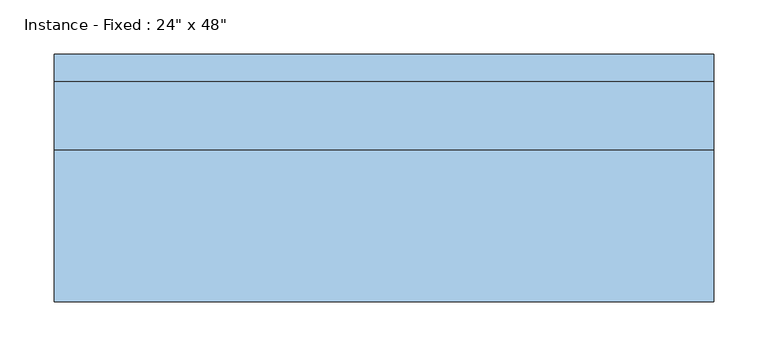
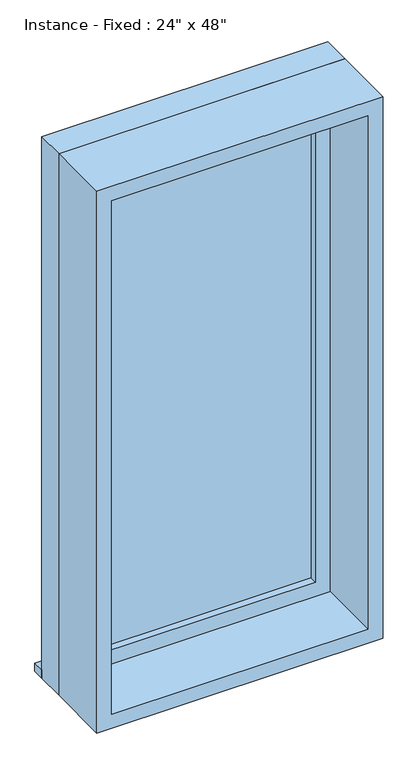
"""IFC4 building model written with IfcOpenShell, lengths in millimetres: window geometry."""

from ifc_helpers import new_model, si_unit, frame, origin, place, context, project, spatial, polyline, outline, extrude, source, transform, mapped, element, save


def window_78885257(model_context):
    return source(origin(), model_context, "Body", "SweptSolid", [
        extrude(outline(polyline([(-342.9, 127.0), (266.7, 127.0), (266.7, 101.6), (-342.9, 101.6), (-342.9, 127.0)])), frame((0.0, 0.0, 914.4), z_axis=(0.0, 0.0, 1.0), x_axis=(1.0, 0.0, 0.0)), (0.0, 0.0, 1.0), 19.05),
        extrude(outline(polyline([(203.2, 53.975), (-279.4, 53.975), (-279.4, 66.675), (203.2, 66.675), (203.2, 53.975)])), frame((0.0, 0.0, 977.9), z_axis=(0.0, 0.0, 1.0), x_axis=(1.0, 0.0, 0.0)), (0.0, 0.0, 1.0), 1092.2),
        extrude(outline(polyline([(2114.55, -323.85), (933.45, -323.85), (933.45, 247.65), (2114.55, 247.65), (2114.55, -323.85)]), holes=[polyline([(2070.1, -279.4), (2070.1, 203.2), (977.9, 203.2), (977.9, -279.4), (2070.1, -279.4)])]), frame((0.0, 38.1, 0.0), z_axis=(0.0, 1.0, 0.0), x_axis=(0.0, 0.0, 1.0)), (0.0, 0.0, 1.0), 44.45),
        extrude(outline(polyline([(2133.6, -342.9), (914.4, -342.9), (914.4, 266.7), (2133.6, 266.7), (2133.6, -342.9)]), holes=[polyline([(2101.85, -311.15), (2101.85, 234.95), (946.15, 234.95), (946.15, -311.15), (2101.85, -311.15)])]), frame((0.0, -101.6, 0.0), z_axis=(0.0, 1.0, 0.0), x_axis=(0.0, 0.0, 1.0)), (0.0, 0.0, 1.0), 139.7),
        extrude(outline(polyline([(2133.6, 266.7), (2133.6, -342.9), (914.4, -342.9), (914.4, 266.7), (2133.6, 266.7)]), holes=[polyline([(2114.55, 247.65), (933.45, 247.65), (933.45, -323.85), (2114.55, -323.85), (2114.55, 247.65)])]), frame((0.0, 38.1, 0.0), z_axis=(0.0, 1.0, 0.0), x_axis=(0.0, 0.0, 1.0)), (0.0, 0.0, 1.0), 63.5),
    ])


if __name__ == "__main__":
    model = new_model("IFC4")
    model_context = context("Model", 3, world=origin())
    ifc_project = project(units=[si_unit("LENGTHUNIT", "METRE", prefix="MILLI")], contexts=[model_context])
    site = spatial("IfcSite", under=ifc_project)
    building = spatial("IfcBuilding", under=site)
    placement = place(None, origin())
    window_shape = window_78885257(model_context)
    element("IfcWindow", 1, ObjectType="Instance - Fixed : 24\" x 48\"", at=placement, inside=building, context=model_context, shape_type="MappedRepresentation", body=[
        mapped(window_shape, transform((0.0, 0.0, 0.0), x_axis=(1.0, 0.0, 0.0), y_axis=(0.0, 1.0, 0.0), z_axis=(0.0, 0.0, 1.0))),
    ])
    save(model, "model.ifc")

# Revit data of these elements
# Type "Instance - Fixed : 24\" x 48\""
#   Type Mark = "19"
#   Construction Type Id = "GSP4R"
#   Assembly Code = "B2020100"
#   Analytic Construction = "1/8 in Pilkington single glazing"
#   Visual Light Transmittance = 0.9
#   Thermal Resistance (R) = 0.8466 (h·ft²·°F)/BTU
#   Solar Heat Gain Coefficient = 0.86
#   Heat Transfer Coefficient (U) = 1.1812 BTU/(h·ft²·°F)
#   Height [instance default] = 4' - 0"
#   Default Sill Height = 3' - 0"
#   Width [instance default] = 2' - 0"
#   Window Inset = 0' - 0 3/4"
#   Define Thermal Properties by = 1
#   Glass Pane Material = Glass
#   Sash Material = Sash
#   Wall Closure = (empty or 0)
# Element 1 (IfcWindow, "Instance - Fixed : 24\" x 48\"")
#   Materials on its faces: "Sash", "Glass"
# Materials
#   "Glass": class "Glass", colour RGB 0 128 192, transparency 0.75, Description = "Soda Lime Glass", Cost = 0
#   "Sash": class "Wood", colour RGB 224 178 126, transparency 0
